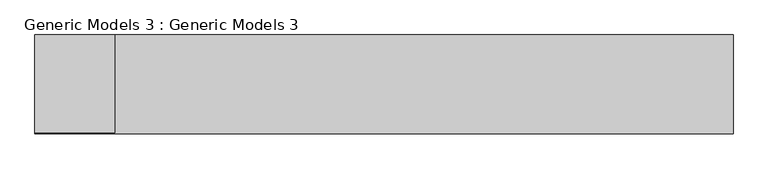
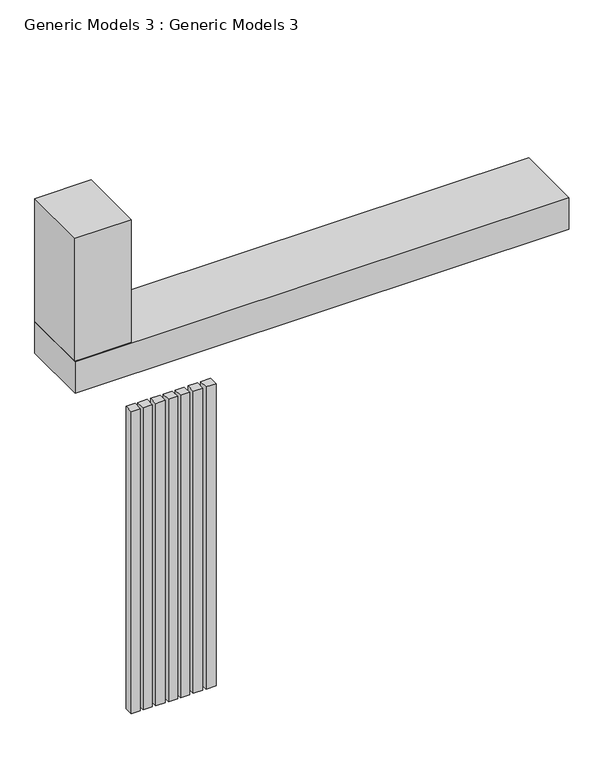
"""IFC4 building model written with IfcOpenShell, lengths in millimetres: proxy geometry, Generic Models 3 : Generic Models 3."""

from ifc_helpers import new_model, si_unit, frame, origin, place, context, project, spatial, polyline, outline, extrude, source, transform, mapped, element, save


def generic_models_3_generic_models_3_6f6c0f21(model_context):
    return source(origin(), model_context, "Body", "SweptSolid", [
        extrude(outline(polyline([(-15444.1837137, -14112.2001929), (-15444.1837137, -14639.6521376), (-15875.429521, -14639.6521376), (-15875.429521, -14112.2001929), (-15444.1837137, -14112.2001929)])), frame((0.0, 0.0, 6654.8), z_axis=(0.0, 0.0, 1.0), x_axis=(1.0, 0.0, 0.0)), (0.0, 0.0, 1.0), 992.2323146),
        extrude(outline(polyline([(-12103.529521, -14645.6001929), (-15875.429521, -14645.6001929), (-15875.429521, -14112.2001929), (-12103.529521, -14112.2001929), (-12103.529521, -14645.6001929)])), frame((0.0, 0.0, 6400.8), z_axis=(0.0, 0.0, 1.0), x_axis=(1.0, 0.0, 0.0)), (0.0, 0.0, 1.0), 254.0),
        extrude(outline(polyline([(-15374.3337137, -14569.8021376), (-15374.3337137, -14639.6521376), (-15444.1837137, -14639.6521376), (-15444.1837137, -14569.8021376), (-15374.3337137, -14569.8021376)])), frame((0.0, 0.0, 3657.6), z_axis=(0.0, 0.0, 1.0), x_axis=(1.0, 0.0, 0.0)), (0.0, 0.0, 1.0), 2438.4),
        extrude(outline(polyline([(-15282.9893332, -14639.6521376), (-15352.9937499, -14639.6521376), (-15352.9937499, -14569.8021376), (-15282.9893332, -14569.8021376), (-15282.9893332, -14639.6521376)])), frame((0.0, 0.0, 3657.6), z_axis=(0.0, 0.0, 1.0), x_axis=(1.0, 0.0, 0.0)), (0.0, 0.0, 1.0), 2438.4),
        extrude(outline(polyline([(-15183.969928, -14639.6521376), (-15256.2771215, -14639.6521376), (-15256.2771215, -14569.8021376), (-15183.969928, -14569.8021376), (-15183.969928, -14639.6521376)])), frame((0.0, 0.0, 3657.6), z_axis=(0.0, 0.0, 1.0), x_axis=(1.0, 0.0, 0.0)), (0.0, 0.0, 1.0), 2438.4),
        extrude(outline(polyline([(-15090.0166319, -14639.6521376), (-15159.5604932, -14639.6521376), (-15159.5604932, -14569.8021376), (-15090.0166319, -14569.8021376), (-15090.0166319, -14639.6521376)])), frame((0.0, 0.0, 3657.6), z_axis=(0.0, 0.0, 1.0), x_axis=(1.0, 0.0, 0.0)), (0.0, 0.0, 1.0), 2438.4),
        extrude(outline(polyline([(-14998.3661127, -14639.6521376), (-15067.4494186, -14639.6521376), (-15067.4494186, -14569.8021376), (-14998.3661127, -14569.8021376), (-14998.3661127, -14639.6521376)])), frame((0.0, 0.0, 3657.6), z_axis=(0.0, 0.0, 1.0), x_axis=(1.0, 0.0, 0.0)), (0.0, 0.0, 1.0), 2438.4),
        extrude(outline(polyline([(-14897.413733, -14639.6521376), (-14969.8947862, -14639.6521376), (-14969.8947862, -14569.8021376), (-14897.413733, -14569.8021376), (-14897.413733, -14639.6521376)])), frame((0.0, 0.0, 3657.6), z_axis=(0.0, 0.0, 1.0), x_axis=(1.0, 0.0, 0.0)), (0.0, 0.0, 1.0), 2438.4),
        extrude(outline(polyline([(-14796.9147937, -14639.6521376), (-14873.0503538, -14639.6521376), (-14873.0503538, -14569.8021376), (-14796.9147937, -14569.8021376), (-14796.9147937, -14639.6521376)])), frame((0.0, 0.0, 3657.6), z_axis=(0.0, 0.0, 1.0), x_axis=(1.0, 0.0, 0.0)), (0.0, 0.0, 1.0), 2438.4),
    ])


if __name__ == "__main__":
    model = new_model("IFC4")
    model_context = context("Model", 3, world=origin())
    ifc_project = project(units=[si_unit("LENGTHUNIT", "METRE", prefix="MILLI")], contexts=[model_context])
    site = spatial("IfcSite", under=ifc_project)
    building = spatial("IfcBuilding", under=site)
    placement = place(None, origin())
    generic_models_3_generic_models_3_shape = generic_models_3_generic_models_3_6f6c0f21(model_context)
    element("IfcBuildingElementProxy", 1, Name="Generic Models 3 : Generic Models 3", ObjectType="Generic Models 3 : Generic Models 3", at=placement, inside=building, context=model_context, shape_type="MappedRepresentation", body=[
        mapped(generic_models_3_generic_models_3_shape, transform((0.0, 0.0, 0.0), x_axis=(1.0, 0.0, 0.0), y_axis=(0.0, 1.0, 0.0), z_axis=(0.0, 0.0, 1.0))),
    ])
    save(model, "model.ifc")
